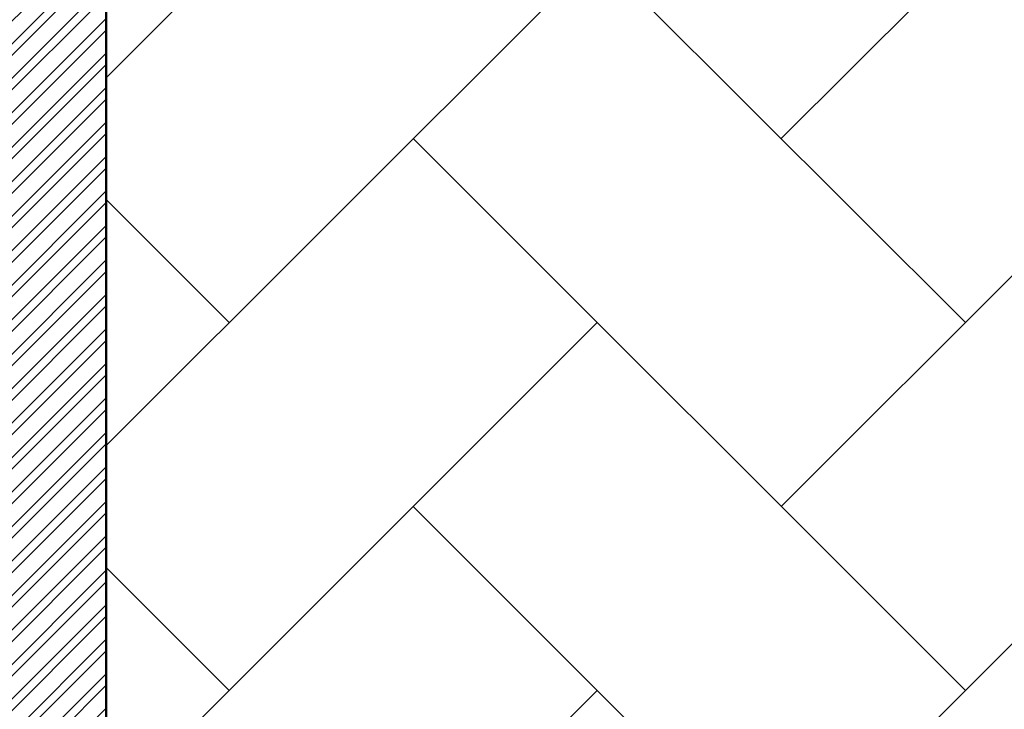
# Model space of a CAD drawing. Units: inches. Extents: x 3590 to 5167, y 65 to 1917.
# Tile 48 of 100: x 4927 to 5003, y 1450 to 1504. Entities that reach past the tile are written whole.
import ezdxf

# ---------------------------------------------------------------- set-up
doc = ezdxf.new("R2010")
doc.units = ezdxf.units.IN
for name, color, linetype, lineweight in [('A-FLOR-PATT', 8, 'Continuous', 13), ('A-WALL', 7, 'Continuous', 50), ('A-WALL-PATT', 251, 'Continuous', 13)]:
    doc.layers.add(name, color=color, linetype=linetype, lineweight=lineweight)

msp = doc.modelspace()

# ---------------------------------------------------------------- hatches: boundary and pattern name
at = {"layer": 'A-FLOR-PATT', "transparency": 33554687}
h = msp.add_hatch(dxfattribs=at)
h.set_pattern_fill('AR-HBONE', color=256, scale=0.2)
h.set_pattern_definition([(45, (-588.972, 0), (0, 28.73682), [60.96, -20.32]), (135, (-574.604, 14.368), (3e-15, 28.73682), [60.96, -20.32])])
h.paths.add_polyline_path([(5071.274, 1796.999), (4933.274, 1796.999), (4933.274, 1753.999), (4962.774, 1753.999, -0.414214), (4928.774, 1719.999), (4933.274, 1718.999), (4933.274, 1334.999), (5071.274, 1334.999)])
h.paths.add_polyline_path([(4951.78, 1521.077), (4951.715, 1521.04), (4951.563, 1520.895)], flags=16)
h.paths.add_polyline_path([(4952.267, 1521.376), (4952.198, 1521.371), (4952.198, 1521.356)], flags=0)
h.paths.add_polyline_path([(4967.051, 1529.728), (4965.231, 1528.694), (4963.411, 1527.714), (4961.756, 1526.851), (4963.589, 1527.449), (4964.036, 1527.478), (4962.975, 1527.249), (4961.76, 1526.852), (4959.792, 1525.834), (4958.005, 1524.895), (4956.24, 1523.93), (4954.504, 1522.919), (4954.129, 1522.682), (4953.361, 1521.997), (4953.366, 1521.998), (4953.605, 1522.064), (4955.106, 1522.761), (4956.921, 1523.434), (4958.678, 1523.915), (4960.358, 1524.2), (4961.945, 1524.286), (4964.171, 1524.108), (4965.958, 1523.309), (4963.863, 1522.976), (4965.187, 1522.499), (4963.366, 1522.497), (4961.545, 1522.487), (4959.764, 1522.461), (4958.304, 1522.419), (4957.974, 1522.388), (4956.307, 1522.232), (4954.718, 1522.071), (4953.251, 1521.899), (4953.525, 1521.623), (4954.331, 1521.379), (4956.243, 1521.23), (4958.039, 1520.93), (4959.684, 1520.483), (4961.16, 1519.896), (4963.107, 1518.8), (4964.393, 1517.325), (4962.973, 1517.726), (4964.558, 1516.661), (4965.407, 1515.708), (4963.507, 1516.322), (4961.68, 1517.005), (4959.935, 1517.745), (4958.282, 1518.528), (4956.732, 1519.343), (4955.295, 1520.175), (4954.672, 1520.572), (4954.513, 1520.627), (4955.658, 1519.318), (4956.703, 1517.982), (4957.644, 1516.647), (4958.485, 1515.334), (4959.55, 1513.524), (4960.438, 1511.769), (4958.841, 1513.62), (4957.452, 1515.325), (4955.819, 1517.459), (4956.665, 1515.448), (4957.111, 1513.923), (4957.447, 1511.714), (4957.076, 1509.793), (4956.538, 1511.11), (4955.992, 1512.569), (4955.444, 1514.125), (4954.898, 1515.735), (4954.357, 1517.356), (4953.824, 1518.943), (4953.305, 1520.452), (4953.065, 1521.116), (4952.971, 1521.146), (4952.949, 1521.086), (4952.73, 1520.199), (4953.37, 1518.024), (4953.757, 1516.373), (4954.051, 1514.765), (4954.264, 1513.221), (4954.471, 1511.131), (4954.497, 1510.402), (4954.409, 1511.76), (4954.264, 1513.221), (4954.051, 1514.765), (4953.757, 1516.373), (4953.37, 1518.024), (4952.877, 1519.698), (4952.716, 1520.141), (4952.533, 1519.059), (4952.374, 1517.789), (4952.219, 1516.312), (4952.046, 1514.6), (4951.833, 1512.626), (4951.557, 1510.363), (4951.203, 1512.168), (4950.852, 1514.339), (4950.985, 1516.376), (4951.66, 1518.286), (4952.593, 1520.481), (4952.357, 1521.13), (4951.855, 1520.328), (4950.839, 1518.908), (4949.777, 1517.587), (4948.916, 1516.617), (4948.111, 1515.256), (4947.089, 1513.554), (4945.889, 1511.615), (4946.326, 1513.402), (4946.562, 1514.249), (4945.528, 1513.327), (4944.581, 1512.531), (4946.018, 1514.508), (4947.204, 1516.048), (4947.893, 1517.313), (4949.307, 1518.764), (4950.414, 1519.767), (4950.451, 1519.806), (4952.267, 1521.376), (4951.645, 1521.493), (4950.404, 1521.18), (4948.044, 1520.359), (4946.119, 1519.452), (4944.572, 1518.475), (4943.35, 1517.443), (4941.997, 1515.92), (4941.661, 1515.275), (4942.813, 1516.99), (4944.572, 1518.475), (4946.119, 1519.452), (4948.044, 1520.359), (4950.404, 1521.18), (4951.645, 1521.493), (4949.647, 1521.868), (4948.6, 1521.756), (4947.126, 1521.57), (4945.42, 1521.348), (4943.45, 1521.105), (4941.183, 1520.856), (4942.86, 1521.613), (4943.873, 1522.03), (4942.952, 1521.909), (4941.41, 1521.485), (4939.543, 1520.67), (4938.968, 1520.226), (4940.733, 1521.299), (4942.952, 1521.909), (4943.702, 1522.008), (4945.894, 1522.7), (4947.565, 1522.714), (4948.921, 1522.566), (4951.131, 1522.183), (4950.971, 1522.297), (4948.129, 1523.006), (4946.035, 1523.707), (4944.232, 1524.521), (4942.707, 1525.461), (4941.444, 1526.537), (4940.43, 1527.761), (4939.649, 1529.143), (4941.421, 1528.122), (4943.147, 1527.132), (4944.841, 1526.175), (4946.514, 1525.25), (4948.179, 1524.359), (4948.365, 1524.263), (4946.475, 1526.045), (4945.181, 1527.54), (4944.19, 1529.033), (4943.496, 1530.54), (4943.278, 1531.36), (4942.498, 1531.919), (4943.114, 1531.762), (4942.959, 1533.659), (4944.14, 1531.989), (4944.612, 1531.323), (4946.202, 1530.463), (4947.486, 1529.509), (4948.79, 1528.226), (4950.368, 1526.237), (4949.485, 1528.155), (4948.851, 1530.123), (4948.491, 1532.041), (4948.381, 1533.918), (4948.501, 1535.76), (4948.827, 1537.573), (4949.418, 1535.565), (4949.957, 1533.569), (4950.464, 1531.586), (4950.961, 1529.617), (4951.391, 1527.954), (4951.724, 1530.687), (4952.201, 1532.58), (4952.889, 1534.33), (4953.77, 1535.951), (4954.827, 1537.46), (4954.521, 1535.39), (4954.273, 1533.937), (4955.58, 1535.663), (4956.748, 1536.739), (4956.159, 1534.78), (4955.589, 1532.873), (4955.043, 1531.006), (4954.525, 1529.166), (4954.038, 1527.341), (4953.638, 1525.733), (4953.611, 1525.586), (4953.398, 1524.166), (4953.382, 1524.009), (4954.07, 1525.476), (4954.912, 1527.022), (4956.136, 1528.894), (4957.847, 1530.577), (4959.376, 1531.54), (4958.256, 1530.104), (4957.143, 1528.663), (4956.066, 1527.243), (4955.056, 1525.871), (4954.141, 1524.571), (4953.352, 1523.372), (4953.311, 1523.303), (4953.273, 1522.925), (4953.261, 1522.382), (4954.103, 1523.373), (4954.63, 1524.284), (4955.961, 1526.358), (4957.23, 1528.13), (4958.421, 1529.609), (4960.037, 1531.368), (4961.374, 1532.375), (4962.101, 1532.77), (4961.07, 1531.061), (4959.987, 1529.438), (4958.869, 1527.908), (4958.15, 1527.007), (4959.803, 1528.003), (4961.589, 1528.793), (4963.391, 1529.328), (4965.211, 1529.632)], flags=16)
h.paths.add_polyline_path([(4962.944, 1523.182), (4961.107, 1523.422), (4960.392, 1523.362), (4962.35, 1523.331)], flags=0)
h.paths.add_polyline_path([(5049.541, 1584.551), (5049.476, 1584.515), (5049.325, 1584.37)], flags=16)
h.paths.add_polyline_path([(5050.028, 1584.851), (5049.959, 1584.845), (5049.959, 1584.83)], flags=0)
h.paths.add_polyline_path([(5042.333, 1581.949), (5043.88, 1582.926), (5045.806, 1583.833), (5048.165, 1584.654), (5049.406, 1584.967), (5047.408, 1585.342), (5046.361, 1585.231), (5044.888, 1585.044), (5043.181, 1584.822), (5041.211, 1584.579), (5038.944, 1584.33), (5040.622, 1585.087), (5041.634, 1585.504), (5040.713, 1585.383), (5039.171, 1584.959), (5037.304, 1584.144), (5036.729, 1583.7), (5038.494, 1584.773), (5040.713, 1585.383), (5041.463, 1585.482), (5043.655, 1586.174), (5045.326, 1586.188), (5046.682, 1586.04), (5048.893, 1585.657), (5048.732, 1585.771), (5045.891, 1586.48), (5043.796, 1587.181), (5041.994, 1587.996), (5040.468, 1588.935), (5039.205, 1590.011), (5038.191, 1591.235), (5037.41, 1592.617), (5039.182, 1591.596), (5040.909, 1590.607), (5042.602, 1589.649), (5044.275, 1588.724), (5045.94, 1587.833), (5046.126, 1587.738), (5044.237, 1589.519), (5042.942, 1591.015), (5041.952, 1592.508), (5041.257, 1594.014), (5041.039, 1594.834), (5040.26, 1595.393), (5040.875, 1595.237), (5040.721, 1597.133), (5041.901, 1595.463), (5042.373, 1594.798), (5043.963, 1593.938), (5045.247, 1592.983), (5046.552, 1591.701), (5048.129, 1589.712), (5047.247, 1591.63), (5046.613, 1593.597), (5046.252, 1595.515), (5046.142, 1597.392), (5046.262, 1599.234), (5046.588, 1601.047), (5047.179, 1599.039), (5047.718, 1597.043), (5048.225, 1595.06), (5048.722, 1593.091), (5049.152, 1591.429), (5049.485, 1594.161), (5049.962, 1596.054), (5050.65, 1597.804), (5051.532, 1599.425), (5052.589, 1600.934), (5052.283, 1598.864), (5052.034, 1597.411), (5053.341, 1599.137), (5054.509, 1600.213), (5053.92, 1598.254), (5053.35, 1596.348), (5052.805, 1594.48), (5052.286, 1592.64), (5051.799, 1590.815), (5051.4, 1589.207), (5051.373, 1589.06), (5051.159, 1587.64), (5051.143, 1587.483), (5051.831, 1588.95), (5052.673, 1590.496), (5053.898, 1592.368), (5055.608, 1594.051), (5057.137, 1595.014), (5056.017, 1593.578), (5054.904, 1592.137), (5053.828, 1590.717), (5052.817, 1589.345), (5051.902, 1588.046), (5051.113, 1586.846), (5051.072, 1586.777), (5051.034, 1586.399), (5051.022, 1585.856), (5051.864, 1586.847), (5052.391, 1587.758), (5053.723, 1589.832), (5054.991, 1591.604), (5056.182, 1593.083), (5057.798, 1594.842), (5059.135, 1595.849), (5059.863, 1596.244), (5058.831, 1594.535), (5057.749, 1592.912), (5056.63, 1591.382), (5055.912, 1590.482), (5057.564, 1591.477), (5059.35, 1592.267), (5061.152, 1592.802), (5062.972, 1593.106), (5064.812, 1593.203), (5062.992, 1592.169), (5061.172, 1591.188), (5059.518, 1590.325), (5061.35, 1590.924), (5061.797, 1590.952), (5060.737, 1590.723), (5059.521, 1590.326), (5057.553, 1589.308), (5055.766, 1588.369), (5054.002, 1587.404), (5052.265, 1586.393), (5051.891, 1586.156), (5051.122, 1585.471), (5051.127, 1585.472), (5051.366, 1585.538), (5052.867, 1586.235), (5054.682, 1586.908), (5056.439, 1587.389), (5058.12, 1587.675), (5059.706, 1587.76), (5061.933, 1587.583), (5063.719, 1586.783), (5061.624, 1586.45), (5062.949, 1585.973), (5061.127, 1585.971), (5059.307, 1585.961), (5057.525, 1585.935), (5056.065, 1585.893), (5055.735, 1585.862), (5054.068, 1585.707), (5052.479, 1585.546), (5051.012, 1585.373), (5051.286, 1585.097), (5052.092, 1584.853), (5054.004, 1584.704), (5055.8, 1584.404), (5057.446, 1583.958), (5058.921, 1583.37), (5060.868, 1582.274), (5062.154, 1580.799), (5060.734, 1581.2), (5062.32, 1580.135), (5063.168, 1579.182), (5061.269, 1579.796), (5059.441, 1580.479), (5057.696, 1581.219), (5056.043, 1582.003), (5054.493, 1582.817), (5053.057, 1583.649), (5052.433, 1584.047), (5052.274, 1584.101), (5053.42, 1582.793), (5054.464, 1581.457), (5055.405, 1580.121), (5056.247, 1578.809), (5057.311, 1576.998), (5058.199, 1575.244), (5056.602, 1577.094), (5055.213, 1578.799), (5053.58, 1580.933), (5054.427, 1578.922), (5054.872, 1577.397), (5055.208, 1575.189), (5054.838, 1573.267), (5054.299, 1574.584), (5053.754, 1576.043), (5053.206, 1577.599), (5052.659, 1579.209), (5052.118, 1580.83), (5051.585, 1582.417), (5051.066, 1583.927), (5050.826, 1584.59), (5050.733, 1584.62), (5050.711, 1584.561), (5050.491, 1583.673), (5051.131, 1581.498), (5051.518, 1579.847), (5051.813, 1578.24), (5052.026, 1576.695), (5052.233, 1574.605), (5052.258, 1573.876), (5052.17, 1575.234), (5052.026, 1576.695), (5051.813, 1578.24), (5051.518, 1579.847), (5051.131, 1581.498), (5050.638, 1583.172), (5050.477, 1583.615), (5050.294, 1582.533), (5050.136, 1581.263), (5049.981, 1579.786), (5049.807, 1578.074), (5049.594, 1576.1), (5049.318, 1573.837), (5048.965, 1575.642), (5048.613, 1577.813), (5048.747, 1579.85), (5049.421, 1581.76), (5050.354, 1583.955), (5050.118, 1584.604), (5049.616, 1583.802), (5048.6, 1582.382), (5047.538, 1581.061), (5046.677, 1580.091), (5045.872, 1578.73), (5044.85, 1577.028), (5043.651, 1575.089), (5044.087, 1576.877), (5044.324, 1577.723), (5043.289, 1576.801), (5042.342, 1576.005), (5043.779, 1577.982), (5044.966, 1579.522), (5045.655, 1580.787), (5047.068, 1582.239), (5048.175, 1583.241), (5048.213, 1583.28), (5050.028, 1584.851), (5049.406, 1584.967), (5048.165, 1584.654), (5045.806, 1583.833), (5043.88, 1582.926), (5042.333, 1581.949), (5041.111, 1580.917), (5039.758, 1579.394), (5039.423, 1578.749), (5040.575, 1580.464)], flags=16)
h.paths.add_polyline_path([(4954.799, 1533.12), (4954.262, 1532.079), (4953.831, 1530.935), (4953.505, 1529.636), (4953.283, 1528.133), (4953.167, 1526.376), (4953.156, 1524.315), (4953.277, 1521.236), (4952.802, 1521.842), (4951.557, 1521.998), (4950.976, 1521.961), (4952.661, 1521.941), (4952.802, 1521.842), (4953.152, 1523.593), (4953.167, 1526.376), (4953.283, 1528.133), (4953.609, 1530.346), (4954.456, 1532.592)], flags=0)
h.paths.add_polyline_path([(5050.563, 1585.316), (5049.318, 1585.472), (5048.737, 1585.435), (5050.422, 1585.415), (5050.563, 1585.316), (5050.914, 1587.067), (5050.928, 1589.851), (5051.045, 1591.607), (5051.371, 1593.82), (5052.217, 1596.066), (5052.56, 1596.594), (5052.024, 1595.554), (5051.592, 1594.409), (5051.266, 1593.11), (5051.045, 1591.607), (5050.928, 1589.851), (5050.918, 1587.789), (5051.038, 1584.71)], flags=0)
h.paths.add_polyline_path([(5058.153, 1586.836), (5060.111, 1586.805), (5060.705, 1586.656), (5058.868, 1586.896)], flags=0)
h.paths.add_polyline_path([(5049.541, 1430.936), (5049.476, 1430.9), (5049.325, 1430.755)], flags=16)
h.paths.add_polyline_path([(5050.028, 1431.236), (5049.959, 1431.231), (5049.959, 1431.215)], flags=0)
h.paths.add_polyline_path([(5046.588, 1447.432), (5047.179, 1445.425), (5047.718, 1443.429), (5048.225, 1441.446), (5048.722, 1439.476), (5049.152, 1437.814), (5049.485, 1440.546), (5049.962, 1442.439), (5050.65, 1444.189), (5051.532, 1445.811), (5052.589, 1447.319), (5052.283, 1445.249), (5052.034, 1443.796), (5053.341, 1445.522), (5054.509, 1446.598), (5053.92, 1444.64), (5053.35, 1442.733), (5052.805, 1440.865), (5052.286, 1439.025), (5051.799, 1437.201), (5051.4, 1435.592), (5051.373, 1435.445), (5051.159, 1434.025), (5051.143, 1433.868), (5051.831, 1435.335), (5052.673, 1436.881), (5053.898, 1438.753), (5055.608, 1440.436), (5057.137, 1441.4), (5056.017, 1439.963), (5054.904, 1438.522), (5053.828, 1437.102), (5052.817, 1435.73), (5051.902, 1434.431), (5051.113, 1433.231), (5051.072, 1433.162), (5051.034, 1432.784), (5051.022, 1432.242), (5051.864, 1433.232), (5052.391, 1434.143), (5053.723, 1436.217), (5054.991, 1437.989), (5056.182, 1439.468), (5057.798, 1441.227), (5059.135, 1442.235), (5059.863, 1442.629), (5058.831, 1440.921), (5057.749, 1439.298), (5056.63, 1437.767), (5055.912, 1436.867), (5057.564, 1437.863), (5059.35, 1438.652), (5061.152, 1439.187), (5062.972, 1439.491), (5064.812, 1439.588), (5062.992, 1438.554), (5061.172, 1437.573), (5059.518, 1436.71), (5061.35, 1437.309), (5061.797, 1437.337), (5060.737, 1437.108), (5059.521, 1436.711), (5057.553, 1435.693), (5055.766, 1434.754), (5054.002, 1433.789), (5052.265, 1432.778), (5051.891, 1432.541), (5051.122, 1431.856), (5051.127, 1431.857), (5051.366, 1431.923), (5052.867, 1432.62), (5054.682, 1433.293), (5056.439, 1433.775), (5058.12, 1434.06), (5059.706, 1434.145), (5061.933, 1433.968), (5063.719, 1433.168), (5061.624, 1432.835), (5062.949, 1432.358), (5061.127, 1432.357), (5059.307, 1432.346), (5057.525, 1432.32), (5056.065, 1432.278), (5055.735, 1432.248), (5054.068, 1432.092), (5052.479, 1431.931), (5051.012, 1431.759), (5051.286, 1431.482), (5052.092, 1431.238), (5054.004, 1431.089), (5055.8, 1430.789), (5057.446, 1430.343), (5058.921, 1429.755), (5060.868, 1428.66), (5062.154, 1427.185), (5060.734, 1427.585), (5062.32, 1426.52), (5063.168, 1425.567), (5061.269, 1426.181), (5059.441, 1426.865), (5057.696, 1427.604), (5056.043, 1428.388), (5054.493, 1429.202), (5053.057, 1430.034), (5052.433, 1430.432), (5052.274, 1430.487), (5053.42, 1429.178), (5054.464, 1427.842), (5055.405, 1426.506), (5056.247, 1425.194), (5057.311, 1423.383), (5058.199, 1421.629), (5056.602, 1423.479), (5055.213, 1425.184), (5053.58, 1427.318), (5054.427, 1425.307), (5054.872, 1423.782), (5055.208, 1421.574), (5054.838, 1419.652), (5054.299, 1420.97), (5053.754, 1422.428), (5053.206, 1423.984), (5052.659, 1425.595), (5052.118, 1427.215), (5051.585, 1428.802), (5051.066, 1430.312), (5050.826, 1430.975), (5050.733, 1431.005), (5050.711, 1430.946), (5050.491, 1430.058), (5051.131, 1427.883), (5051.518, 1426.232), (5051.813, 1424.625), (5052.026, 1423.081), (5052.233, 1420.991), (5052.258, 1420.261), (5052.17, 1421.619), (5052.026, 1423.081), (5051.813, 1424.625), (5051.518, 1426.232), (5051.131, 1427.883), (5050.638, 1429.558), (5050.477, 1430.001), (5050.294, 1428.918), (5050.136, 1427.648), (5049.981, 1426.171), (5049.807, 1424.459), (5049.594, 1422.485), (5049.318, 1420.222), (5048.965, 1422.028), (5048.613, 1424.199), (5048.747, 1426.235), (5049.421, 1428.146), (5050.354, 1430.34), (5050.118, 1430.989), (5049.616, 1430.187), (5048.6, 1428.768), (5047.538, 1427.446), (5046.677, 1426.477), (5045.872, 1425.116), (5044.85, 1423.413), (5043.651, 1421.474), (5044.087, 1423.262), (5044.324, 1424.109), (5043.289, 1423.186), (5042.342, 1422.391), (5043.779, 1424.368), (5044.966, 1425.907), (5045.655, 1427.173), (5047.068, 1428.624), (5048.175, 1429.627), (5048.213, 1429.666), (5050.028, 1431.236), (5049.406, 1431.353), (5048.165, 1431.039), (5045.806, 1430.218), (5043.88, 1429.311), (5042.333, 1428.334), (5041.111, 1427.302), (5039.758, 1425.779), (5039.423, 1425.134), (5040.575, 1426.849), (5042.333, 1428.334), (5043.88, 1429.311), (5045.806, 1430.218), (5048.165, 1431.039), (5049.406, 1431.353), (5047.408, 1431.727), (5046.361, 1431.616), (5044.888, 1431.429), (5043.181, 1431.207), (5041.211, 1430.964), (5038.944, 1430.715), (5040.622, 1431.472), (5041.634, 1431.89), (5040.713, 1431.769), (5039.171, 1431.345), (5037.304, 1430.53), (5036.729, 1430.085), (5038.494, 1431.158), (5040.713, 1431.769), (5041.463, 1431.867), (5043.655, 1432.559), (5045.326, 1432.573), (5046.682, 1432.425), (5048.893, 1432.042), (5048.732, 1432.156), (5045.891, 1432.865), (5043.796, 1433.566), (5041.994, 1434.381), (5040.468, 1435.321), (5039.205, 1436.396), (5038.191, 1437.62), (5037.41, 1439.002), (5039.182, 1437.982), (5040.909, 1436.992), (5042.602, 1436.034), (5044.275, 1435.109), (5045.94, 1434.218), (5046.126, 1434.123), (5044.237, 1435.904), (5042.942, 1437.4), (5041.952, 1438.893), (5041.257, 1440.399), (5041.039, 1441.219), (5040.26, 1441.778), (5040.875, 1441.622), (5040.721, 1443.518), (5041.901, 1441.848), (5042.373, 1441.183), (5043.963, 1440.323), (5045.247, 1439.369), (5046.552, 1438.086), (5048.129, 1436.097), (5047.247, 1438.015), (5046.613, 1439.982), (5046.252, 1441.901), (5046.142, 1443.778), (5046.262, 1445.619)], flags=16)
h.paths.add_polyline_path([(5052.382, 1444.255), (5051.623, 1442.78), (5052.024, 1441.939), (5052.56, 1442.98)], flags=0)
h.paths.add_polyline_path([(5050.563, 1431.701), (5049.318, 1431.857), (5048.737, 1431.821), (5050.422, 1431.8)], flags=0)
h.paths.add_polyline_path([(5058.153, 1433.221), (5060.111, 1433.19), (5060.705, 1433.041), (5058.868, 1433.281)], flags=0)
h.paths.add_polyline_path([(5049.541, 1352.285), (5049.476, 1352.249), (5049.325, 1352.104)], flags=16)
h.paths.add_polyline_path([(5050.028, 1352.585), (5049.959, 1352.58), (5049.959, 1352.564)], flags=0)
h.paths.add_polyline_path([(5046.588, 1368.781), (5047.179, 1366.774), (5047.718, 1364.778), (5048.225, 1362.795), (5048.722, 1360.825), (5049.152, 1359.163), (5049.485, 1361.896), (5049.962, 1363.789), (5050.65, 1365.538), (5051.532, 1367.16), (5052.589, 1368.669), (5052.283, 1366.598), (5052.034, 1365.145), (5053.341, 1366.871), (5054.509, 1367.947), (5053.92, 1365.989), (5053.35, 1364.082), (5052.805, 1362.214), (5052.286, 1360.374), (5051.799, 1358.55), (5051.4, 1356.942), (5051.373, 1356.794), (5051.159, 1355.374), (5051.143, 1355.218), (5051.831, 1356.684), (5052.673, 1358.23), (5053.898, 1360.102), (5055.608, 1361.786), (5057.137, 1362.749), (5056.017, 1361.313), (5054.904, 1359.872), (5053.828, 1358.452), (5052.817, 1357.079), (5051.902, 1355.78), (5051.113, 1354.581), (5051.072, 1354.512), (5051.034, 1354.133), (5051.022, 1353.591), (5051.864, 1354.581), (5052.391, 1355.492), (5053.723, 1357.566), (5054.991, 1359.338), (5056.182, 1360.817), (5057.798, 1362.577), (5059.135, 1363.584), (5059.863, 1363.979), (5058.831, 1362.27), (5057.749, 1360.647), (5056.63, 1359.117), (5055.912, 1358.216), (5057.564, 1359.212), (5059.35, 1360.001), (5061.152, 1360.536), (5062.972, 1360.841), (5064.812, 1360.937), (5062.992, 1359.903), (5061.172, 1358.923), (5059.518, 1358.059), (5061.35, 1358.658), (5061.797, 1358.687), (5060.737, 1358.458), (5059.521, 1358.061), (5057.553, 1357.043), (5055.766, 1356.103), (5054.002, 1355.138), (5052.265, 1354.127), (5051.891, 1353.89), (5051.122, 1353.206), (5051.127, 1353.206), (5051.366, 1353.272), (5052.867, 1353.969), (5054.682, 1354.643), (5056.439, 1355.124), (5058.12, 1355.409), (5059.706, 1355.495), (5061.933, 1355.317), (5063.719, 1354.518), (5061.624, 1354.184), (5062.949, 1353.708), (5061.127, 1353.706), (5059.307, 1353.695), (5057.525, 1353.669), (5056.065, 1353.627), (5055.735, 1353.597), (5054.068, 1353.441), (5052.479, 1353.28), (5051.012, 1353.108), (5051.286, 1352.831), (5052.092, 1352.587), (5054.004, 1352.439), (5055.8, 1352.138), (5057.446, 1351.692), (5058.921, 1351.104), (5060.868, 1350.009), (5062.154, 1348.534), (5060.734, 1348.935), (5062.32, 1347.869), (5063.168, 1346.916), (5061.269, 1347.53), (5059.441, 1348.214), (5057.696, 1348.954), (5056.043, 1349.737), (5054.493, 1350.551), (5053.057, 1351.383), (5052.433, 1351.781), (5052.274, 1351.836), (5053.42, 1350.527), (5054.464, 1349.191), (5055.405, 1347.855), (5056.247, 1346.543), (5057.311, 1344.733), (5058.199, 1342.978), (5056.602, 1344.828), (5055.213, 1346.534), (5053.58, 1348.667), (5054.427, 1346.656), (5054.872, 1345.132), (5055.208, 1342.923), (5054.838, 1341.002), (5054.299, 1342.319), (5053.754, 1343.778), (5053.206, 1345.334), (5052.659, 1346.944), (5052.118, 1348.564), (5051.585, 1350.151), (5051.066, 1351.661), (5050.826, 1352.324), (5050.733, 1352.355), (5050.711, 1352.295), (5050.491, 1351.408), (5051.131, 1349.232), (5051.518, 1347.581), (5051.813, 1345.974), (5052.026, 1344.43), (5052.233, 1342.34), (5052.258, 1341.61), (5052.17, 1342.969), (5052.026, 1344.43), (5051.813, 1345.974), (5051.518, 1347.581), (5051.131, 1349.232), (5050.638, 1350.907), (5050.477, 1351.35), (5050.294, 1350.267), (5050.136, 1348.997), (5049.981, 1347.52), (5049.807, 1345.809), (5049.594, 1343.835), (5049.318, 1341.571), (5048.965, 1343.377), (5048.613, 1345.548), (5048.747, 1347.585), (5049.421, 1349.495), (5050.354, 1351.689), (5050.118, 1352.339), (5049.616, 1351.536), (5048.6, 1350.117), (5047.538, 1348.795), (5046.677, 1347.826), (5045.872, 1346.465), (5044.85, 1344.763), (5043.651, 1342.824), (5044.087, 1344.611), (5044.324, 1345.458), (5043.289, 1344.535), (5042.342, 1343.74), (5043.779, 1345.717), (5044.966, 1347.256), (5045.655, 1348.522), (5047.068, 1349.973), (5048.175, 1350.976), (5048.213, 1351.015), (5050.028, 1352.585), (5049.406, 1352.702), (5048.165, 1352.388), (5045.806, 1351.567), (5043.88, 1350.661), (5042.333, 1349.683), (5041.111, 1348.651), (5039.758, 1347.128), (5039.423, 1346.483), (5040.575, 1348.198), (5042.333, 1349.683), (5043.88, 1350.661), (5045.806, 1351.567), (5048.165, 1352.388), (5049.406, 1352.702), (5047.408, 1353.076), (5046.361, 1352.965), (5044.888, 1352.779), (5043.181, 1352.556), (5041.211, 1352.313), (5038.944, 1352.065), (5040.622, 1352.821), (5041.634, 1353.239), (5040.713, 1353.118), (5039.171, 1352.694), (5037.304, 1351.879), (5036.729, 1351.434), (5038.494, 1352.508), (5040.713, 1353.118), (5041.463, 1353.216), (5043.655, 1353.909), (5045.326, 1353.923), (5046.682, 1353.774), (5048.893, 1353.391), (5048.732, 1353.506), (5045.891, 1354.214), (5043.796, 1354.915), (5041.994, 1355.73), (5040.468, 1356.67), (5039.205, 1357.746), (5038.191, 1358.969), (5037.41, 1360.352), (5039.182, 1359.331), (5040.909, 1358.341), (5042.602, 1357.383), (5044.275, 1356.458), (5045.94, 1355.567), (5046.126, 1355.472), (5044.237, 1357.253), (5042.942, 1358.749), (5041.952, 1360.242), (5041.257, 1361.748), (5041.039, 1362.568), (5040.26, 1363.128), (5040.875, 1362.971), (5040.721, 1364.867), (5041.901, 1363.197), (5042.373, 1362.532), (5043.963, 1361.672), (5045.247, 1360.718), (5046.552, 1359.435), (5048.129, 1357.446), (5047.247, 1359.364), (5046.613, 1361.331), (5046.252, 1363.25), (5046.142, 1365.127), (5046.262, 1366.969)], flags=16)
h.paths.add_polyline_path([(5052.382, 1365.604), (5051.623, 1364.129), (5052.024, 1363.288), (5052.56, 1364.329)], flags=0)
h.paths.add_polyline_path([(4951.78, 1698.041), (4951.715, 1698.005), (4951.563, 1697.859)], flags=16)
h.paths.add_polyline_path([(4952.267, 1698.341), (4952.198, 1698.335), (4952.198, 1698.32)], flags=0)
h.paths.add_polyline_path([(4957.076, 1686.757), (4956.538, 1688.074), (4955.992, 1689.533), (4955.444, 1691.089), (4954.898, 1692.699), (4954.357, 1694.32), (4953.824, 1695.907), (4953.305, 1697.417), (4953.065, 1698.08), (4952.971, 1698.11), (4952.949, 1698.051), (4952.73, 1697.163), (4953.37, 1694.988), (4953.757, 1693.337), (4954.051, 1691.729), (4954.264, 1690.185), (4954.471, 1688.095), (4954.497, 1687.366), (4954.409, 1688.724), (4954.264, 1690.185), (4954.051, 1691.729), (4953.757, 1693.337), (4953.37, 1694.988), (4952.877, 1696.662), (4952.716, 1697.105), (4952.533, 1696.023), (4952.374, 1694.753), (4952.219, 1693.276), (4952.046, 1691.564), (4951.833, 1689.59), (4951.557, 1687.327), (4951.203, 1689.132), (4950.852, 1691.303), (4950.985, 1693.34), (4951.66, 1695.25), (4952.593, 1697.445), (4952.357, 1698.094), (4951.855, 1697.292), (4950.839, 1695.872), (4949.777, 1694.551), (4948.916, 1693.581), (4948.111, 1692.22), (4947.089, 1690.518), (4945.889, 1688.579), (4946.326, 1690.366), (4946.562, 1691.213), (4945.528, 1690.291), (4944.581, 1689.495), (4946.018, 1691.472), (4947.204, 1693.012), (4947.893, 1694.277), (4949.307, 1695.729), (4950.414, 1696.731), (4950.451, 1696.77), (4952.267, 1698.341), (4951.645, 1698.457), (4950.404, 1698.144), (4948.044, 1697.323), (4946.119, 1696.416), (4944.572, 1695.439), (4943.35, 1694.407), (4941.997, 1692.884), (4941.661, 1692.239), (4942.813, 1693.954), (4944.572, 1695.439), (4946.119, 1696.416), (4948.044, 1697.323), (4950.404, 1698.144), (4951.645, 1698.457), (4949.647, 1698.832), (4948.6, 1698.72), (4947.126, 1698.534), (4945.42, 1698.312), (4943.45, 1698.069), (4941.183, 1697.82), (4942.86, 1698.577), (4943.873, 1698.994), (4942.952, 1698.873), (4941.41, 1698.449), (4939.543, 1697.634), (4938.968, 1697.19), (4940.733, 1698.263), (4942.952, 1698.873), (4943.702, 1698.972), (4945.894, 1699.664), (4947.565, 1699.678), (4948.921, 1699.53), (4951.131, 1699.147), (4950.971, 1699.261), (4948.129, 1699.97), (4946.035, 1700.671), (4944.232, 1701.486), (4942.707, 1702.425), (4941.444, 1703.501), (4940.43, 1704.725), (4939.649, 1706.107), (4941.421, 1705.086), (4943.147, 1704.097), (4944.841, 1703.139), (4946.514, 1702.214), (4948.179, 1701.323), (4948.365, 1701.227), (4946.475, 1703.009), (4945.181, 1704.505), (4944.19, 1705.997), (4943.496, 1707.504), (4943.278, 1708.324), (4942.498, 1708.883), (4943.114, 1708.727), (4942.959, 1710.623), (4944.14, 1708.953), (4944.612, 1708.287), (4946.202, 1707.428), (4947.486, 1706.473), (4948.79, 1705.191), (4950.368, 1703.202), (4949.485, 1705.12), (4948.851, 1707.087), (4948.491, 1709.005), (4948.381, 1710.882), (4948.501, 1712.724), (4948.827, 1714.537), (4949.418, 1712.529), (4949.957, 1710.533), (4950.464, 1708.55), (4950.961, 1706.581), (4951.391, 1704.919), (4951.724, 1707.651), (4952.201, 1709.544), (4952.889, 1711.294), (4953.77, 1712.915), (4954.827, 1714.424), (4954.521, 1712.354), (4954.273, 1710.901), (4955.58, 1712.627), (4956.748, 1713.703), (4956.159, 1711.744), (4955.589, 1709.837), (4955.043, 1707.97), (4954.525, 1706.13), (4954.038, 1704.305), (4953.638, 1702.697), (4953.611, 1702.55), (4953.398, 1701.13), (4953.382, 1700.973), (4954.07, 1702.44), (4954.912, 1703.986), (4956.136, 1705.858), (4957.847, 1707.541), (4959.376, 1708.504), (4958.256, 1707.068), (4957.143, 1705.627), (4956.066, 1704.207), (4955.056, 1702.835), (4954.141, 1701.536), (4953.352, 1700.336), (4953.311, 1700.267), (4953.273, 1699.889), (4953.261, 1699.346), (4954.103, 1700.337), (4954.63, 1701.248), (4955.961, 1703.322), (4957.23, 1705.094), (4958.421, 1706.573), (4960.037, 1708.332), (4961.374, 1709.339), (4962.101, 1709.734), (4961.07, 1708.025), (4959.987, 1706.402), (4958.869, 1704.872), (4958.15, 1703.972), (4959.803, 1704.967), (4961.589, 1705.757), (4963.391, 1706.292), (4965.211, 1706.596), (4967.051, 1706.692), (4965.231, 1705.659), (4963.411, 1704.678), (4961.756, 1703.815), (4963.589, 1704.413), (4964.036, 1704.442), (4962.975, 1704.213), (4961.76, 1703.816), (4959.792, 1702.798), (4958.005, 1701.859), (4956.24, 1700.894), (4954.504, 1699.883), (4954.129, 1699.646), (4953.361, 1698.961), (4953.366, 1698.962), (4953.605, 1699.028), (4955.106, 1699.725), (4956.921, 1700.398), (4958.678, 1700.879), (4960.358, 1701.164), (4961.945, 1701.25), (4964.171, 1701.073), (4965.958, 1700.273), (4963.863, 1699.94), (4965.187, 1699.463), (4963.366, 1699.461), (4961.545, 1699.451), (4959.764, 1699.425), (4958.304, 1699.383), (4957.974, 1699.352), (4956.307, 1699.197), (4954.718, 1699.036), (4953.251, 1698.863), (4953.525, 1698.587), (4954.331, 1698.343), (4956.243, 1698.194), (4958.039, 1697.894), (4959.684, 1697.447), (4961.16, 1696.86), (4963.107, 1695.764), (4964.393, 1694.289), (4962.973, 1694.69), (4964.558, 1693.625), (4965.407, 1692.672), (4963.507, 1693.286), (4961.68, 1693.969), (4959.935, 1694.709), (4958.282, 1695.492), (4956.732, 1696.307), (4955.295, 1697.139), (4954.672, 1697.536), (4954.513, 1697.591), (4955.658, 1696.282), (4956.703, 1694.946), (4957.644, 1693.611), (4958.485, 1692.298), (4959.55, 1690.488), (4960.438, 1688.733), (4958.841, 1690.584), (4957.452, 1692.289), (4955.819, 1694.423), (4956.665, 1692.412), (4957.111, 1690.887), (4957.447, 1688.678)], flags=16)
h.paths.add_polyline_path([(5050.563, 1353.05), (5049.318, 1353.207), (5048.737, 1353.17), (5050.422, 1353.15)], flags=0)
h.paths.add_polyline_path([(4951.78, 1351.486), (4951.715, 1351.45), (4951.563, 1351.305)], flags=16)
h.paths.add_polyline_path([(4952.267, 1351.786), (4952.198, 1351.78), (4952.198, 1351.765)], flags=0)
h.paths.add_polyline_path([(4954.827, 1367.869), (4954.521, 1365.799), (4954.273, 1364.346), (4955.58, 1366.072), (4956.748, 1367.148), (4956.159, 1365.19), (4955.589, 1363.283), (4955.043, 1361.415), (4954.525, 1359.575), (4954.038, 1357.751), (4953.638, 1356.142), (4953.611, 1355.995), (4953.398, 1354.575), (4953.382, 1354.418), (4954.07, 1355.885), (4954.912, 1357.431), (4956.136, 1359.303), (4957.847, 1360.986), (4959.376, 1361.95), (4958.256, 1360.513), (4957.143, 1359.072), (4956.066, 1357.652), (4955.056, 1356.28), (4954.141, 1354.981), (4953.352, 1353.781), (4953.311, 1353.712), (4953.273, 1353.334), (4953.261, 1352.792), (4954.103, 1353.782), (4954.63, 1354.693), (4955.961, 1356.767), (4957.23, 1358.539), (4958.421, 1360.018), (4960.037, 1361.777), (4961.374, 1362.785), (4962.101, 1363.179), (4961.07, 1361.471), (4959.987, 1359.848), (4958.869, 1358.317), (4958.15, 1357.417), (4959.803, 1358.413), (4961.589, 1359.202), (4963.391, 1359.737), (4965.211, 1360.041), (4967.051, 1360.138), (4965.231, 1359.104), (4963.411, 1358.123), (4961.756, 1357.26), (4963.589, 1357.859), (4964.036, 1357.887), (4962.975, 1357.658), (4961.76, 1357.261), (4959.792, 1356.243), (4958.005, 1355.304), (4956.24, 1354.339), (4954.504, 1353.328), (4954.129, 1353.091), (4953.361, 1352.406), (4953.366, 1352.407), (4953.605, 1352.473), (4955.106, 1353.17), (4956.921, 1353.843), (4958.678, 1354.325), (4960.358, 1354.61), (4961.945, 1354.695), (4964.171, 1354.518), (4965.958, 1353.718), (4963.863, 1353.385), (4965.187, 1352.908), (4963.366, 1352.907), (4961.545, 1352.896), (4959.764, 1352.87), (4958.304, 1352.828), (4957.974, 1352.798), (4956.307, 1352.642), (4954.718, 1352.481), (4953.251, 1352.309), (4953.525, 1352.032), (4954.331, 1351.788), (4956.243, 1351.639), (4958.039, 1351.339), (4959.684, 1350.893), (4961.16, 1350.305), (4963.107, 1349.21), (4964.393, 1347.735), (4962.973, 1348.135), (4964.558, 1347.07), (4965.407, 1346.117), (4963.507, 1346.731), (4961.68, 1347.414), (4959.935, 1348.154), (4958.282, 1348.938), (4956.732, 1349.752), (4955.295, 1350.584), (4954.672, 1350.982), (4954.513, 1351.036), (4955.658, 1349.728), (4956.703, 1348.392), (4957.644, 1347.056), (4958.485, 1345.744), (4959.55, 1343.933), (4960.438, 1342.179), (4958.841, 1344.029), (4957.452, 1345.734), (4955.819, 1347.868), (4956.665, 1345.857), (4957.111, 1344.332), (4957.447, 1342.124), (4957.076, 1340.202), (4956.538, 1341.52), (4955.992, 1342.978), (4955.444, 1344.534), (4954.898, 1346.145), (4954.357, 1347.765), (4953.824, 1349.352), (4953.305, 1350.862), (4953.065, 1351.525), (4952.971, 1351.555), (4952.949, 1351.496), (4952.73, 1350.608), (4953.37, 1348.433), (4953.757, 1346.782), (4954.051, 1345.175), (4954.264, 1343.631), (4954.471, 1341.541), (4954.497, 1340.811), (4954.409, 1342.169), (4954.264, 1343.631), (4954.051, 1345.175), (4953.757, 1346.782), (4953.37, 1348.433), (4952.877, 1350.108), (4952.716, 1350.551), (4952.533, 1349.468), (4952.374, 1348.198), (4952.219, 1346.721), (4952.046, 1345.009), (4951.833, 1343.035), (4951.557, 1340.772), (4951.203, 1342.578), (4950.852, 1344.749), (4950.985, 1346.785), (4951.66, 1348.696), (4952.593, 1350.89), (4952.357, 1351.539), (4951.855, 1350.737), (4950.839, 1349.318), (4949.777, 1347.996), (4948.916, 1347.027), (4948.111, 1345.665), (4947.089, 1343.963), (4945.889, 1342.024), (4946.326, 1343.812), (4946.562, 1344.659), (4945.528, 1343.736), (4944.581, 1342.941), (4946.018, 1344.918), (4947.204, 1346.457), (4947.893, 1347.723), (4949.307, 1349.174), (4950.414, 1350.177), (4950.451, 1350.216), (4952.267, 1351.786), (4951.645, 1351.903), (4950.404, 1351.589), (4948.044, 1350.768), (4946.119, 1349.861), (4944.572, 1348.884), (4943.35, 1347.852), (4941.997, 1346.329), (4941.661, 1345.684), (4942.813, 1347.399), (4944.572, 1348.884), (4946.119, 1349.861), (4948.044, 1350.768), (4950.404, 1351.589), (4951.645, 1351.903), (4949.647, 1352.277), (4948.6, 1352.166), (4947.126, 1351.979), (4945.42, 1351.757), (4943.45, 1351.514), (4941.183, 1351.265), (4942.86, 1352.022), (4943.873, 1352.44), (4942.952, 1352.319), (4941.41, 1351.895), (4939.543, 1351.08), (4938.968, 1350.635), (4940.733, 1351.708), (4942.952, 1352.319), (4943.702, 1352.417), (4945.894, 1353.109), (4947.565, 1353.123), (4948.921, 1352.975), (4951.131, 1352.592), (4950.971, 1352.706), (4948.129, 1353.415), (4946.035, 1354.116), (4944.232, 1354.931), (4942.707, 1355.871), (4941.444, 1356.946), (4940.43, 1358.17), (4939.649, 1359.552), (4941.421, 1358.532), (4943.147, 1357.542), (4944.841, 1356.584), (4946.514, 1355.659), (4948.179, 1354.768), (4948.365, 1354.673), (4946.475, 1356.454), (4945.181, 1357.95), (4944.19, 1359.443), (4943.496, 1360.949), (4943.278, 1361.769), (4942.498, 1362.328), (4943.114, 1362.172), (4942.959, 1364.068), (4944.14, 1362.398), (4944.612, 1361.733), (4946.202, 1360.873), (4947.486, 1359.919), (4948.79, 1358.636), (4950.368, 1356.647), (4949.485, 1358.565), (4948.851, 1360.532), (4948.491, 1362.451), (4948.381, 1364.328), (4948.501, 1366.169), (4948.827, 1367.982), (4949.418, 1365.975), (4949.957, 1363.979), (4950.464, 1361.995), (4950.961, 1360.026), (4951.391, 1358.364), (4951.724, 1361.096), (4952.201, 1362.989), (4952.889, 1364.739), (4953.77, 1366.361)], flags=16)
h.paths.add_polyline_path([(4954.799, 1363.53), (4954.262, 1362.489), (4953.831, 1361.344), (4953.505, 1360.045), (4953.283, 1358.543), (4953.167, 1356.786), (4953.156, 1354.724), (4953.277, 1351.646), (4952.802, 1352.251), (4951.557, 1352.407), (4950.976, 1352.371), (4952.661, 1352.35), (4952.802, 1352.251), (4953.152, 1354.002), (4953.167, 1356.786), (4953.283, 1358.543), (4953.609, 1360.755), (4954.456, 1363.001)], flags=0)
h.paths.add_polyline_path([(4952.802, 1698.806), (4951.557, 1698.962), (4950.976, 1698.925), (4952.661, 1698.905), (4952.802, 1698.806), (4953.152, 1700.557), (4953.167, 1703.34), (4953.283, 1705.097), (4953.609, 1707.31), (4954.456, 1709.556), (4954.799, 1710.084), (4954.262, 1709.043), (4953.831, 1707.899), (4953.505, 1706.6), (4953.283, 1705.097), (4953.167, 1703.34), (4953.156, 1701.279), (4953.277, 1698.2)], flags=0)
h.paths.add_polyline_path([(4962.944, 1700.146), (4961.107, 1700.386), (4960.392, 1700.326), (4962.35, 1700.295)], flags=0)
h.paths.add_polyline_path([(5058.153, 1354.57), (5060.111, 1354.539), (5060.705, 1354.391), (5058.868, 1354.631)], flags=0)
h.paths.add_polyline_path([(4962.944, 1353.591), (4961.107, 1353.831), (4960.392, 1353.771), (4962.35, 1353.74)], flags=0)
h.paths.add_polyline_path([(5049.541, 1778.72), (5049.476, 1778.684), (5049.325, 1778.539)], flags=16)
h.paths.add_polyline_path([(5050.028, 1779.02), (5049.959, 1779.014), (5049.959, 1778.999)], flags=0)
h.paths.add_polyline_path([(5052.258, 1768.045), (5052.17, 1769.403), (5052.026, 1770.864), (5051.813, 1772.409), (5051.518, 1774.016), (5051.131, 1775.667), (5050.638, 1777.341), (5050.477, 1777.784), (5050.294, 1776.702), (5050.136, 1775.432), (5049.981, 1773.955), (5049.807, 1772.243), (5049.594, 1770.269), (5049.318, 1768.006), (5048.965, 1769.811), (5048.613, 1771.982), (5048.747, 1774.019), (5049.421, 1775.929), (5050.354, 1778.124), (5050.118, 1778.773), (5049.616, 1777.971), (5048.6, 1776.551), (5047.538, 1775.23), (5046.677, 1774.26), (5045.872, 1772.899), (5044.85, 1771.197), (5043.651, 1769.258), (5044.087, 1771.046), (5044.324, 1771.892), (5043.289, 1770.97), (5042.342, 1770.174), (5043.779, 1772.151), (5044.966, 1773.691), (5045.655, 1774.956), (5047.068, 1776.408), (5048.175, 1777.41), (5048.213, 1777.449), (5050.028, 1779.02), (5049.406, 1779.136), (5048.165, 1778.823), (5045.806, 1778.002), (5043.88, 1777.095), (5042.333, 1776.118), (5041.111, 1775.086), (5039.758, 1773.563), (5039.423, 1772.918), (5040.575, 1774.633), (5042.333, 1776.118), (5043.88, 1777.095), (5045.806, 1778.002), (5048.165, 1778.823), (5049.406, 1779.136), (5047.408, 1779.511), (5046.361, 1779.4), (5044.888, 1779.213), (5043.181, 1778.991), (5041.211, 1778.748), (5038.944, 1778.499), (5040.622, 1779.256), (5041.634, 1779.673), (5040.713, 1779.552), (5039.171, 1779.128), (5037.304, 1778.313), (5036.729, 1777.869), (5038.494, 1778.942), (5040.713, 1779.552), (5041.463, 1779.651), (5043.655, 1780.343), (5045.326, 1780.357), (5046.682, 1780.209), (5048.893, 1779.826), (5048.732, 1779.94), (5045.891, 1780.649), (5043.796, 1781.35), (5041.994, 1782.165), (5040.468, 1783.104), (5039.205, 1784.18), (5038.191, 1785.404), (5037.41, 1786.786), (5039.182, 1785.765), (5040.909, 1784.776), (5042.602, 1783.818), (5044.275, 1782.893), (5045.94, 1782.002), (5046.126, 1781.907), (5044.237, 1783.688), (5042.942, 1785.184), (5041.952, 1786.677), (5041.257, 1788.183), (5041.039, 1789.003), (5040.26, 1789.562), (5040.875, 1789.406), (5040.721, 1791.302), (5041.901, 1789.632), (5042.373, 1788.967), (5043.963, 1788.107), (5045.247, 1787.152), (5046.552, 1785.87), (5048.129, 1783.881), (5047.247, 1785.799), (5046.613, 1787.766), (5046.252, 1789.684), (5046.142, 1791.561), (5046.262, 1793.403), (5046.588, 1795.216), (5047.179, 1793.208), (5047.718, 1791.213), (5048.225, 1789.229), (5048.722, 1787.26), (5049.152, 1785.598), (5049.485, 1788.33), (5049.962, 1790.223), (5050.65, 1791.973), (5051.532, 1793.594), (5052.589, 1795.103), (5052.283, 1793.033), (5052.034, 1791.58), (5053.341, 1793.306), (5054.509, 1794.382), (5053.92, 1792.423), (5053.35, 1790.517), (5052.805, 1788.649), (5052.286, 1786.809), (5051.799, 1784.984), (5051.4, 1783.376), (5051.373, 1783.229), (5051.159, 1781.809), (5051.143, 1781.652), (5051.831, 1783.119), (5052.673, 1784.665), (5053.898, 1786.537), (5055.608, 1788.22), (5057.137, 1789.183), (5056.017, 1787.747), (5054.904, 1786.306), (5053.828, 1784.886), (5052.817, 1783.514), (5051.902, 1782.215), (5051.113, 1781.015), (5051.072, 1780.946), (5051.034, 1780.568), (5051.022, 1780.025), (5051.864, 1781.016), (5052.391, 1781.927), (5053.723, 1784.001), (5054.991, 1785.773), (5056.182, 1787.252), (5057.798, 1789.011), (5059.135, 1790.018), (5059.863, 1790.413), (5058.831, 1788.704), (5057.749, 1787.081), (5056.63, 1785.551), (5055.912, 1784.651), (5057.564, 1785.646), (5059.35, 1786.436), (5061.152, 1786.971), (5062.972, 1787.275), (5064.812, 1787.372), (5062.992, 1786.338), (5061.172, 1785.357), (5059.518, 1784.494), (5061.35, 1785.093), (5061.797, 1785.121), (5060.737, 1784.892), (5059.521, 1784.495), (5057.553, 1783.477), (5055.766, 1782.538), (5054.002, 1781.573), (5052.265, 1780.562), (5051.891, 1780.325), (5051.122, 1779.64), (5051.127, 1779.641), (5051.366, 1779.707), (5052.867, 1780.404), (5054.682, 1781.077), (5056.439, 1781.558), (5058.12, 1781.844), (5059.706, 1781.929), (5061.933, 1781.752), (5063.719, 1780.952), (5061.624, 1780.619), (5062.949, 1780.142), (5061.127, 1780.14), (5059.307, 1780.13), (5057.525, 1780.104), (5056.065, 1780.062), (5055.735, 1780.031), (5054.068, 1779.876), (5052.479, 1779.715), (5051.012, 1779.542), (5051.286, 1779.266), (5052.092, 1779.022), (5054.004, 1778.873), (5055.8, 1778.573), (5057.446, 1778.127), (5058.921, 1777.539), (5060.868, 1776.443), (5062.154, 1774.968), (5060.734, 1775.369), (5062.32, 1774.304), (5063.168, 1773.351), (5061.269, 1773.965), (5059.441, 1774.648), (5057.696, 1775.388), (5056.043, 1776.172), (5054.493, 1776.986), (5053.057, 1777.818), (5052.433, 1778.216), (5052.274, 1778.27), (5053.42, 1776.962), (5054.464, 1775.626), (5055.405, 1774.29), (5056.247, 1772.978), (5057.311, 1771.167), (5058.199, 1769.413), (5056.602, 1771.263), (5055.213, 1772.968), (5053.58, 1775.102), (5054.427, 1773.091), (5054.872, 1771.566), (5055.208, 1769.358), (5054.838, 1767.436), (5054.299, 1768.753), (5053.754, 1770.212), (5053.206, 1771.768), (5052.659, 1773.378), (5052.118, 1774.999), (5051.585, 1776.586), (5051.066, 1778.096), (5050.826, 1778.759), (5050.733, 1778.789), (5050.711, 1778.73), (5050.491, 1777.842), (5051.131, 1775.667), (5051.518, 1774.016), (5051.813, 1772.409), (5052.026, 1770.864), (5052.233, 1768.774)], flags=16)
h.paths.add_polyline_path([(5050.563, 1779.485), (5049.318, 1779.641), (5048.737, 1779.604), (5050.422, 1779.584), (5050.563, 1779.485), (5050.914, 1781.236), (5050.928, 1784.02), (5051.045, 1785.776), (5051.371, 1787.989), (5052.217, 1790.235), (5052.56, 1790.763), (5052.024, 1789.723), (5051.592, 1788.578), (5051.266, 1787.279), (5051.045, 1785.776), (5050.928, 1784.02), (5050.918, 1781.958), (5051.038, 1778.879)], flags=0)
h.paths.add_polyline_path([(5058.153, 1781.005), (5060.111, 1780.974), (5060.705, 1780.825), (5058.868, 1781.065)], flags=0)
at = {"layer": 'A-WALL-PATT', "transparency": 33554687}
h = msp.add_hatch(dxfattribs=at)
h.set_pattern_fill('ANSI32', color=256, scale=0.2)
h.paths.add_polyline_path([(4684.274, 1805.999), (4591.274, 1805.999), (4591.274, 1796.999), (4639.274, 1796.999), (4639.274, 1790.999), (4648.274, 1790.999), (4648.274, 1796.999), (4684.274, 1796.999)])
h.paths.add_polyline_path([(4543.274, 1805.999), (4420.274, 1805.999), (4420.274, 1784.999), (4429.274, 1784.999), (4429.274, 1796.999), (4445.919, 1796.999), (4543.274, 1796.999)])
h.paths.add_polyline_path([(4828.274, 1805.999), (4744.274, 1805.999), (4744.274, 1796.999), (4828.274, 1796.999)])
h.paths.add_polyline_path([(4648.274, 1754.999), (4639.274, 1754.999), (4639.274, 1655.999), (4546.274, 1655.999), (4546.274, 1649.999), (4549.274, 1649.999), (4549.274, 1553.999), (4429.274, 1553.999), (4429.274, 1583.999), (4420.274, 1583.999), (4420.274, 1538.999), (4429.274, 1538.999), (4429.274, 1544.999), (4639.274, 1544.999), (4639.274, 1538.999), (4648.274, 1538.999), (4648.274, 1559.999), (4639.274, 1559.999), (4639.274, 1553.999), (4555.274, 1553.999), (4555.274, 1649.999), (4639.274, 1649.999), (4639.274, 1589.999), (4648.274, 1589.999)])
h.paths.add_polyline_path([(4516.274, 1655.999), (4429.274, 1655.999), (4429.274, 1736.999), (4420.274, 1736.999), (4420.274, 1619.999), (4429.274, 1619.999), (4429.274, 1649.999), (4516.274, 1649.999)], flags=17)
h.paths.add_polyline_path([(5080.274, 1805.999), (4888.274, 1805.999), (4888.274, 1796.999), (4924.274, 1796.999), (4924.274, 1754.999), (4933.274, 1754.999), (4933.274, 1796.999), (5071.274, 1796.999), (5071.274, 1334.999), (4933.274, 1334.999), (4933.274, 1565.999), (4924.274, 1565.999), (4924.274, 1334.999), (4898.774, 1334.999), (4898.774, 1325.999), (5080.274, 1325.999)])
h.paths.add_polyline_path([(4933.274, 1718.999), (4924.274, 1718.999), (4924.274, 1637.999), (4933.274, 1637.999)], flags=17)
h.paths.add_polyline_path([(4802.774, 1334.999), (4777.274, 1334.999), (4777.274, 1502.999), (4756.274, 1502.999), (4756.274, 1493.999), (4768.274, 1493.999), (4768.274, 1430.999), (4696.274, 1430.999), (4696.274, 1493.999), (4708.274, 1493.999), (4708.274, 1502.999), (4639.274, 1502.999), (4639.274, 1493.999), (4687.274, 1493.999), (4687.274, 1430.999), (4681.274, 1430.999), (4681.274, 1421.999), (4768.274, 1421.999), (4768.274, 1334.999), (4726.274, 1334.999), (4726.274, 1325.999), (4802.774, 1325.999)])
h.paths.add_polyline_path([(4690.274, 1334.999), (4648.274, 1334.999), (4648.274, 1352.867), (4648.274, 1421.999), (4651.274, 1421.999), (4651.274, 1430.999), (4639.274, 1430.999), (4639.274, 1334.999), (4633.274, 1334.999), (4633.274, 1325.999), (4690.274, 1325.999)])
h.paths.add_polyline_path([(4585.274, 1334.999), (4584.724, 1334.999), (4429.274, 1334.999), (4429.274, 1490.999), (4420.274, 1490.999), (4420.274, 1325.999), (4585.274, 1325.999)])

# ---------------------------------------------------------------- linework, layer by layer
at = {"layer": 'A-WALL'}
msp.add_line((4933.274, 1334.999), (4933.274, 1718.999), dxfattribs=at)

doc.saveas('drawing.dxf')
